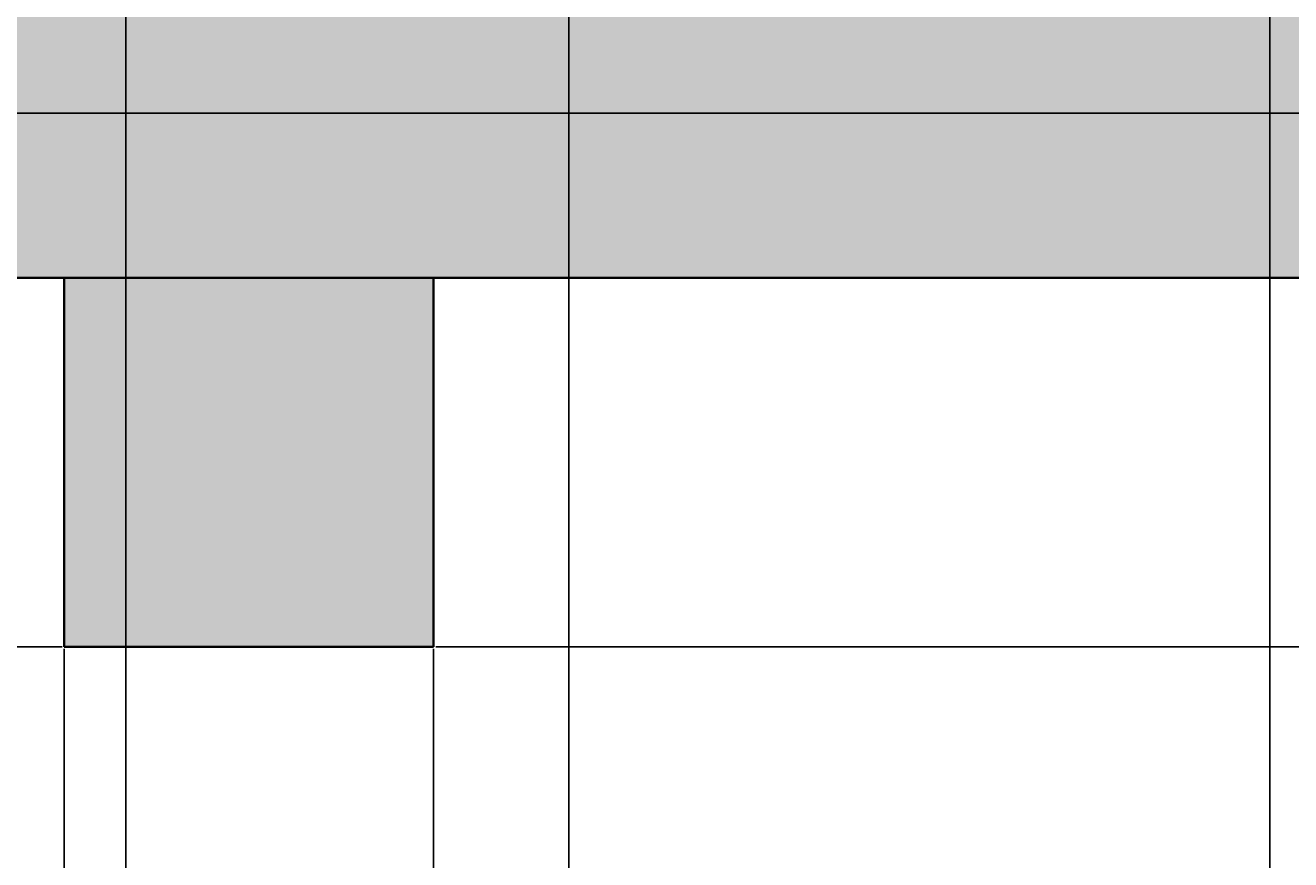
# Model space of a CAD drawing. Units: inches. Extents: x -1 to 292, y -3 to 199.
# Tile 14 of 52: x 68 to 102, y 20 to 42. Entities that reach past the tile are written whole.
import ezdxf

# ---------------------------------------------------------------- set-up
doc = ezdxf.new("R2010")
doc.units = ezdxf.units.IN
doc.header["$MEASUREMENT"] = 0
for name, color, linetype, lineweight in [('M-DIMS', 2, 'Continuous', 18), ('M-EQPM', 7, 'Continuous', 35), ('M-PATT', 8, 'Continuous', 13)]:
    doc.layers.add(name, color=color, linetype=linetype, lineweight=lineweight)
doc.styles.get("Standard").update_dxf_attribs({"font": 'arial.ttf'})
doc.dimstyles.get("Standard").update_dxf_attribs({"dimtxt": 0.18, "dimasz": 0.18, "dimexe": 0.18, "dimexo": 0.0625, "dimgap": 0.09, "dimtad": 0, "dimtih": 1, "dimtoh": 1, "dimdec": 4, "dimzin": 0, "dimdsep": 46, "dimtxsty": 'Standard', "dimcen": 0.09, "dimadec": 0, "dimazin": 0, "dimtfac": 1, "dimtdec": 4, "dimtofl": 0, "dimtmove": 0, "dimatfit": 3, "dimfxl": 1, "dimtolj": 1, "dimtzin": 0, "dimarcsym": 0})

# ---------------------------------------------------------------- blocks, each defined once
blk = doc.blocks.new('SADDLE-SUPPORT')
for p, q in [((0, 10), (0, 0)), ((10, 0), (10, 10)), ((0, 0), (10, 0))]:
    blk.add_line(p, q)
blk = doc.blocks.new('*D7')
at = {"layer": 'Defpoints', "color": 0, "transparency": 16777216}
for p in [(21.861, 54.582), (205.115, 54.582), (21.861, 39.982)]:
    blk.add_point(p, dxfattribs=at)
at = {"layer": 'M-DIMS', "color": 0, "lineweight": -2, "transparency": 16777216}
for p, q in [((21.861, 54.52), (21.861, 39.802)), ((205.115, 54.52), (205.115, 39.802)), ((22.041, 39.982), (113.033, 39.982)), ((204.935, 39.982), (113.944, 39.982))]:
    blk.add_line(p, q, dxfattribs=at)
at = {"layer": 'M-DIMS', "color": 0, "transparency": 16777216}
for points in [[(22.041, 40.012), (22.041, 39.952), (21.861, 39.982)], [(204.935, 40.012), (204.935, 39.952), (205.115, 39.982)]]:
    blk.add_solid(points, dxfattribs=at)
at = {"layer": 'M-DIMS', "color": 0, "transparency": 16777216, "insert": (113.488, 39.982), "char_height": 0.18, "attachment_point": 5}
blk.add_mtext('\\A1;183.25', dxfattribs=at)
blk = doc.blocks.new('*D8')
at = {"layer": 'Defpoints', "color": 0, "transparency": 16777216}
for p in [(-0.662, 126.765), (111.488, 126.765), (69.013, 25.514)]:
    blk.add_point(p, dxfattribs=at)
at = {"layer": 'M-DIMS', "color": 0, "lineweight": -2, "transparency": 16777216}
for p, q in [((111.426, 126.765), (-0.842, 126.765)), ((-0.662, 126.585), (-0.662, 76.321)), ((-0.662, 25.694), (-0.662, 75.958)), ((68.951, 25.514), (-0.842, 25.514))]:
    blk.add_line(p, q, dxfattribs=at)
at = {"layer": 'M-DIMS', "color": 0, "transparency": 16777216}
for points in [[(-0.692, 126.585), (-0.632, 126.585), (-0.662, 126.765)], [(-0.692, 25.694), (-0.632, 25.694), (-0.662, 25.514)]]:
    blk.add_solid(points, dxfattribs=at)
at = {"layer": 'M-DIMS', "color": 0, "transparency": 16777216, "insert": (-0.662, 76.14), "char_height": 0.18, "attachment_point": 5}
blk.add_mtext('\\A1;101.25', dxfattribs=at)
blk = doc.blocks.new('*D11')
at = {"layer": 'Defpoints', "color": 0, "transparency": 16777216}
for p in [(79.013, 35.514), (292.04, 35.514), (79.013, 25.514)]:
    blk.add_point(p, dxfattribs=at)
at = {"layer": 'M-DIMS', "color": 0, "lineweight": -2, "transparency": 16777216}
for p, q in [((79.076, 35.514), (292.22, 35.514)), ((292.04, 35.334), (292.04, 30.696)), ((292.04, 25.694), (292.04, 30.332)), ((79.076, 25.514), (292.22, 25.514))]:
    blk.add_line(p, q, dxfattribs=at)
at = {"layer": 'M-DIMS', "color": 0, "transparency": 16777216}
for points in [[(292.01, 35.334), (292.07, 35.334), (292.04, 35.514)], [(292.01, 25.694), (292.07, 25.694), (292.04, 25.514)]]:
    blk.add_solid(points, dxfattribs=at)
at = {"layer": 'M-DIMS', "color": 0, "transparency": 16777216, "insert": (292.04, 30.514), "char_height": 0.18, "attachment_point": 5}
blk.add_mtext('\\A1;10', dxfattribs=at)
blk = doc.blocks.new('*D12')
at = {"layer": 'Defpoints', "color": 0, "transparency": 16777216}
for p in [(69.013, 25.514), (79.013, 25.514), (69.013, 10.914)]:
    blk.add_point(p, dxfattribs=at)
at = {"layer": 'M-DIMS', "color": 0, "lineweight": -2, "transparency": 16777216}
for p, q in [((69.013, 25.452), (69.013, 10.734)), ((79.013, 25.452), (79.013, 10.734)), ((69.193, 10.914), (73.803, 10.914)), ((78.833, 10.914), (74.223, 10.914))]:
    blk.add_line(p, q, dxfattribs=at)
at = {"layer": 'M-DIMS', "color": 0, "transparency": 16777216}
for points in [[(69.193, 10.944), (69.193, 10.884), (69.013, 10.914)], [(78.833, 10.944), (78.833, 10.884), (79.013, 10.914)]]:
    blk.add_solid(points, dxfattribs=at)
at = {"layer": 'M-DIMS', "color": 0, "transparency": 16777216, "insert": (74.013, 10.914), "char_height": 0.18, "attachment_point": 5}
blk.add_mtext('\\A1;10', dxfattribs=at)
blk = doc.blocks.new('*D13')
at = {"layer": 'Defpoints', "color": 0, "transparency": 16777216}
for p in [(79.013, 25.514), (148.429, 25.514), (79.013, 10.914)]:
    blk.add_point(p, dxfattribs=at)
at = {"layer": 'M-DIMS', "color": 0, "lineweight": -2, "transparency": 16777216}
for p, q in [((79.013, 25.452), (79.013, 10.734)), ((148.429, 25.452), (148.429, 10.734)), ((79.193, 10.914), (113.328, 10.914)), ((148.249, 10.914), (114.115, 10.914))]:
    blk.add_line(p, q, dxfattribs=at)
at = {"layer": 'M-DIMS', "color": 0, "transparency": 16777216}
for points in [[(79.193, 10.944), (79.193, 10.884), (79.013, 10.914)], [(148.249, 10.944), (148.249, 10.884), (148.429, 10.914)]]:
    blk.add_solid(points, dxfattribs=at)
at = {"layer": 'M-DIMS', "color": 0, "transparency": 16777216, "insert": (113.721, 10.914), "char_height": 0.18, "attachment_point": 5}
blk.add_mtext('\\A1;69.42', dxfattribs=at)
blk = doc.blocks.new('*D20')
at = {"layer": 'Defpoints', "color": 0, "transparency": 16777216}
for p in [(64.679, 51.267), (70.679, 51.267), (70.679, -2.71)]:
    blk.add_point(p, dxfattribs=at)
at = {"layer": 'M-DIMS', "color": 0, "lineweight": -2, "transparency": 16777216}
for p, q in [((64.679, 51.205), (64.679, -2.89)), ((70.679, 51.205), (70.679, -2.89)), ((64.859, -2.71), (67.529, -2.71)), ((70.499, -2.71), (67.828, -2.71))]:
    blk.add_line(p, q, dxfattribs=at)
at = {"layer": 'M-DIMS', "color": 0, "transparency": 16777216}
for points in [[(64.859, -2.68), (64.859, -2.74), (64.679, -2.71)], [(70.499, -2.68), (70.499, -2.74), (70.679, -2.71)]]:
    blk.add_solid(points, dxfattribs=at)
at = {"layer": 'M-DIMS', "color": 0, "transparency": 16777216, "insert": (67.679, -2.71), "char_height": 0.18, "attachment_point": 5}
blk.add_mtext('\\A1;6', dxfattribs=at)
blk = doc.blocks.new('*D21')
at = {"layer": 'Defpoints', "color": 0, "transparency": 16777216}
for p in [(82.679, 51.267), (101.679, 51.267), (101.679, -2.71)]:
    blk.add_point(p, dxfattribs=at)
at = {"layer": 'M-DIMS', "color": 0, "lineweight": -2, "transparency": 16777216}
for p, q in [((82.679, 51.205), (82.679, -2.89)), ((101.679, 51.205), (101.679, -2.89)), ((82.859, -2.71), (91.968, -2.71)), ((101.499, -2.71), (92.389, -2.71))]:
    blk.add_line(p, q, dxfattribs=at)
at = {"layer": 'M-DIMS', "color": 0, "transparency": 16777216}
for points in [[(82.859, -2.68), (82.859, -2.74), (82.679, -2.71)], [(101.499, -2.68), (101.499, -2.74), (101.679, -2.71)]]:
    blk.add_solid(points, dxfattribs=at)
at = {"layer": 'M-DIMS', "color": 0, "transparency": 16777216, "insert": (92.179, -2.71), "char_height": 0.18, "attachment_point": 5}
blk.add_mtext('\\A1;19', dxfattribs=at)
blk = doc.blocks.new('*D22')
at = {"layer": 'Defpoints', "color": 0, "transparency": 16777216}
for p in [(82.679, 51.267), (122.679, 51.267), (122.679, -2.71)]:
    blk.add_point(p, dxfattribs=at)
at = {"layer": 'M-DIMS', "color": 0, "lineweight": -2, "transparency": 16777216}
for p, q in [((82.679, 51.205), (82.679, -2.89)), ((122.679, 51.205), (122.679, -2.89)), ((82.859, -2.71), (102.457, -2.71)), ((122.499, -2.71), (102.901, -2.71))]:
    blk.add_line(p, q, dxfattribs=at)
at = {"layer": 'M-DIMS', "color": 0, "transparency": 16777216}
for points in [[(82.859, -2.68), (82.859, -2.74), (82.679, -2.71)], [(122.499, -2.68), (122.499, -2.74), (122.679, -2.71)]]:
    blk.add_solid(points, dxfattribs=at)
at = {"layer": 'M-DIMS', "color": 0, "transparency": 16777216, "insert": (102.679, -2.71), "char_height": 0.18, "attachment_point": 5}
blk.add_mtext('\\A1;40', dxfattribs=at)

msp = doc.modelspace()

# ---------------------------------------------------------------- hatches: boundary and pattern name
at = {"layer": 'M-PATT'}
h = msp.add_hatch(color=256, dxfattribs=at)
h.set_gradient(color1=(0, 255, 255), color2=(0, 255, 255), tint=1)
h.paths.add_polyline_path([(75.3521, 99.7735), (72.66, 101.3278), (70.2665, 99.7735), (67.5744, 101.3278), (65.1809, 99.7735), (62.4888, 101.3278), (60.0953, 99.7735), (57.4032, 101.3278), (55.0097, 99.7735), (52.3176, 101.3278), (49.9241, 99.7735, 0.4142136), (57.8007, 91.897), (61.6788, 91.897), (61.6788, 51.2672), (57.8007, 51.2672, 0.8088808), (54.5813, 36.2021), (65.0947, 51.2672), (64.6788, 51.2672), (64.6788, 91.897), (67.6788, 91.897), (67.6788, 51.2672), (65.0947, 51.2672), (54.5813, 36.2021, 0.1056561), (57.8007, 35.5141), (169.176, 35.5141, 1), (169.176, 51.2672), (162.6788, 51.2672), (162.6788, 91.897), (169.176, 91.897, 0.4144629), (177.0526, 99.7802), (174.372, 101.3278), (171.9786, 99.7735), (169.2864, 101.3278), (166.893, 99.7735), (164.2008, 101.3278), (162.1623, 100.004), (162.1623, 96.1027), (160.6222, 96.1027), (160.6222, 100.4578), (159.1152, 101.3278), (156.7218, 99.7735), (154.0296, 101.3278), (151.6362, 99.7735), (148.944, 101.3278), (146.5506, 99.7735), (143.8584, 101.3278), (141.465, 99.7735), (138.7728, 101.3278), (136.3794, 99.7735), (133.6872, 101.3278), (131.2938, 99.7735), (128.6016, 101.3278), (126.2082, 99.7735), (123.516, 101.3278), (121.1225, 99.7735), (118.4304, 101.3278), (116.0369, 99.7735), (113.3448, 101.3278), (110.9513, 99.7735), (108.2592, 101.3278), (105.8657, 99.7735), (103.1736, 101.3278), (100.7801, 99.7735), (98.088, 101.3278), (95.6945, 99.7735), (93.0024, 101.3278), (90.6089, 99.7735), (87.9168, 101.3278), (85.5233, 99.7735), (82.8312, 101.3278), (80.4377, 99.7735), (77.7456, 101.3278)])
h.paths.add_polyline_path([(79.6788, 91.897), (79.6788, 51.2672), (76.6788, 51.2672), (76.6788, 91.897)], flags=16)
h.paths.add_polyline_path([(73.6788, 91.897), (73.6788, 51.2672), (70.6788, 51.2672), (70.6788, 91.897)], flags=16)
h.paths.add_polyline_path([(82.6788, 91.897), (101.6788, 91.897), (101.6788, 51.2672), (82.6788, 51.2672)], flags=16)
h.paths.add_polyline_path([(104.6788, 91.897), (107.6788, 91.897), (107.6788, 51.2672), (104.6788, 51.2672)], flags=16)
h.paths.add_polyline_path([(110.6788, 91.897), (113.6788, 91.897), (113.6788, 51.2672), (110.6788, 51.2672)], flags=16)
h.paths.add_polyline_path([(116.6788, 91.897), (119.6788, 91.897), (119.6788, 51.2672), (116.6788, 51.2672)], flags=16)
h.paths.add_polyline_path([(122.6788, 91.897), (141.6788, 91.897), (141.6788, 51.2672), (144.6788, 51.2672), (144.6788, 91.897), (147.6788, 91.897), (147.6788, 51.2672), (122.6788, 51.2672)], flags=16)
h.paths.add_polyline_path([(150.6788, 91.897), (153.6788, 91.897), (153.6788, 51.2672), (150.6788, 51.2672)], flags=16)
h.paths.add_polyline_path([(156.6788, 91.897), (159.6788, 91.897), (159.6788, 51.2672), (156.6788, 51.2672)], flags=16)
h = msp.add_hatch(color=256, dxfattribs=at)
h.set_gradient(color1=(128, 128, 128), color2=(192, 192, 192), tint=1, name='CYLINDER')
h.paths.add_polyline_path([(158.4295, 25.5141), (158.4295, 35.5141), (148.4295, 35.5141), (148.4295, 25.5141)])
h.paths.add_polyline_path([(79.013, 25.5141), (79.013, 35.5141), (69.013, 35.5141), (69.013, 25.5141)])
h.paths.add_polyline_path([(253.2006, 30.7296), (249.5623, 37.0313, -0.2494892), (240.7896, 35.6769), (237.9333, 30.7296)])

# ---------------------------------------------------------------- linework, layer by layer
at = {"layer": 'M-EQPM'}
msp.add_lwpolyline([(61.6788, 51.2672), (57.8007, 51.2672, 1), (57.8007, 35.5141), (169.176, 35.5141, 1), (169.176, 51.2672), (162.6788, 51.2672)], format="xyb", dxfattribs=at)

# ---------------------------------------------------------------- block references
msp.add_blockref('SADDLE-SUPPORT', (69.013, 25.514), dxfattribs=at)

# ---------------------------------------------------------------- dimensions: what is measured, and where the dimension line sits
at = {"layer": 'M-DIMS'}
for base, p1, p2, angle, override, picture, middle in [((-0.6625, 126.765), (69.013, 25.5141), (111.4883, 126.765), 90, {"dimdec": 2, "dimlfac": 1, "dimrnd": 0, "dimzin": 0, "dimdsep": 46, "dimlunit": 2}, '*D8', (-0.6625, 76.1396)), ((21.8612, 39.9821), (205.1155, 54.5821), (21.8612, 54.5821), 180, {"dimdec": 2, "dimlfac": 1, "dimrnd": 0, "dimzin": 0, "dimdsep": 46, "dimlunit": 2}, '*D7', (113.4883, 39.9821)), ((292.0399, 35.5141), (79.013, 25.5141), (79.013, 35.5141), 90, {"dimdec": 0, "dimlfac": 1, "dimrnd": 0, "dimzin": 0, "dimdsep": 46, "dimlunit": 2}, '*D11', (292.0399, 30.5141)), ((69.013, 10.9141), (79.013, 25.5141), (69.013, 25.5141), 180, {"dimdec": 0, "dimlfac": 1, "dimrnd": 0, "dimzin": 0, "dimdsep": 46, "dimlunit": 2}, '*D12', (74.013, 10.9141)), ((79.013, 10.9141), (148.4295, 25.5141), (79.013, 25.5141), 180, {"dimdec": 2, "dimlfac": 1, "dimrnd": 0, "dimzin": 0, "dimdsep": 46, "dimlunit": 2}, '*D13', (113.7212, 10.9141))]:
    dim = msp.add_linear_dim(base=base, p1=p1, p2=p2, angle=angle, dimstyle='Standard', override=override, dxfattribs=at)
    dim.commit()
    dim.dimension.update_dxf_attribs({"geometry": picture, "text_midpoint": middle})
for base, p1, p2, picture, middle in [((70.6788, -2.7104), (64.6788, 51.2672), (70.6788, 51.2672), '*D20', (67.6788, -2.7104)), ((101.6788, -2.7104), (82.6788, 51.2672), (101.6788, 51.2672), '*D21', (92.1788, -2.7104)), ((122.6788, -2.7104), (82.6788, 51.2672), (122.6788, 51.2672), '*D22', (102.6788, -2.7104))]:
    dim = msp.add_linear_dim(base=base, p1=p1, p2=p2, dimstyle='Standard', override={"dimdec": 0, "dimlfac": 1, "dimrnd": 0, "dimzin": 0, "dimdsep": 46, "dimlunit": 2}, dxfattribs=at)
    dim.commit()
    dim.dimension.update_dxf_attribs({"geometry": picture, "text_midpoint": middle})

doc.saveas('drawing.dxf')
